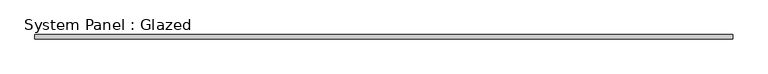
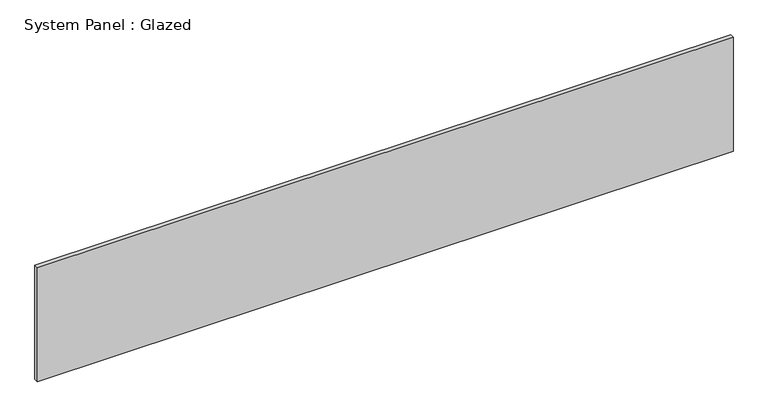
"""IFC4 building model written with IfcOpenShell, lengths in millimetres: plate geometry, System Panel : Glazed."""

from ifc_helpers import new_model, si_unit, origin, origin_with_axes, place, context, project, spatial, polyline, outline, extrude, source, transform, mapped, element, save


def system_panel_glazed_4f9242a6(model_context):
    return source(origin(), model_context, "Body", "SweptSolid", [
        extrude(outline(polyline([(2089.15, 19.05), (-2089.15, 19.05), (-2089.15, 44.45), (2089.15, 44.45), (2089.15, 19.05)])), origin_with_axes(), (0.0, 0.0, 1.0), 724.313055),
    ])


if __name__ == "__main__":
    model = new_model("IFC4")
    model_context = context("Model", 3, world=origin())
    ifc_project = project(units=[si_unit("LENGTHUNIT", "METRE", prefix="MILLI")], contexts=[model_context])
    site = spatial("IfcSite", under=ifc_project)
    building = spatial("IfcBuilding", under=site)
    placement = place(None, origin())
    system_panel_glazed_shape = system_panel_glazed_4f9242a6(model_context)
    element("IfcPlate", 1, ObjectType="System Panel : Glazed", at=placement, inside=building, context=model_context, shape_type="MappedRepresentation", body=[
        mapped(system_panel_glazed_shape, transform((0.0, 0.0, 0.0), x_axis=(1.0, 0.0, 0.0), y_axis=(0.0, 1.0, 0.0), z_axis=(0.0, 0.0, 1.0))),
    ])
    save(model, "model.ifc")

# Revit data of these elements
# Type "System Panel : Glazed"
#   Construction Type Id = "GSP4R"
#   Analytic Construction = "1/8 in Pilkington single glazing"
#   Visual Light Transmittance = 0.9
#   Solar Heat Gain Coefficient = 0.86
#   Heat Transfer Coefficient (U) = 1.18115 BTU/(h·ft²·°F)
#   Define Thermal Properties by = 1
# Element 1 (IfcPlate, "System Panel : Glazed")
#   Materials on its faces: "Glass"
# Materials
#   "Glass": class "Glass", colour RGB 0 128 192, transparency 0.75, Description = "Soda Lime Glass", Cost = 0
